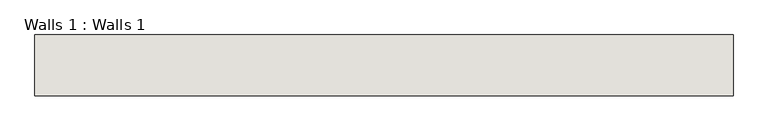
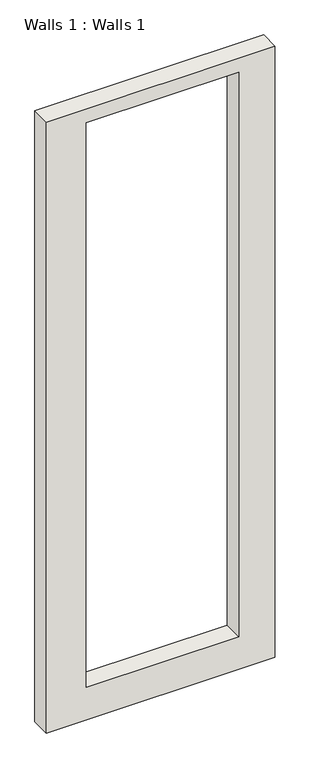
"""IFC4 building model written with IfcOpenShell, lengths in millimetres: wall geometry, Walls 1 : Walls 1."""

from ifc_helpers import new_model, si_unit, frame, origin, place, context, project, spatial, polyline, outline, extrude, source, transform, mapped, element, save


def walls_1_walls_1_c9c6bd33(model_context):
    return source(origin(), model_context, "Body", "SweptSolid", [
        extrude(outline(polyline([(14859.0, -6861.632922), (14859.0, -10366.832922), (4953.0, -10366.832922), (4953.0, -6861.632922), (14859.0, -6861.632922)]), holes=[polyline([(14630.4, -7420.432922), (5486.4, -7420.432922), (5486.4, -9757.232922), (14630.4, -9757.232922), (14630.4, -7420.432922)])]), frame((0.0, 4379.6617654, 0.0), z_axis=(0.0, 1.0, 0.0), x_axis=(0.0, 0.0, 1.0)), (0.0, 0.0, 1.0), 304.8),
    ])


if __name__ == "__main__":
    model = new_model("IFC4")
    model_context = context("Model", 3, world=origin())
    ifc_project = project(units=[si_unit("LENGTHUNIT", "METRE", prefix="MILLI")], contexts=[model_context])
    site = spatial("IfcSite", under=ifc_project)
    building = spatial("IfcBuilding", under=site)
    placement = place(None, origin())
    walls_1_walls_1_shape = walls_1_walls_1_c9c6bd33(model_context)
    element("IfcWall", 1, ObjectType="Walls 1 : Walls 1", at=placement, inside=building, context=model_context, shape_type="MappedRepresentation", body=[
        mapped(walls_1_walls_1_shape, transform((0.0, 0.0, 0.0), x_axis=(1.0, 0.0, 0.0), y_axis=(0.0, 1.0, 0.0), z_axis=(0.0, 0.0, 1.0))),
    ])
    save(model, "model.ifc")

# Revit data of these elements
# Element 1 (IfcWall, "Walls 1 : Walls 1")
#   Materials on its faces: "Default Wall"
# Materials
#   "Default Wall": colour RGB 128 128 128, transparency 0
